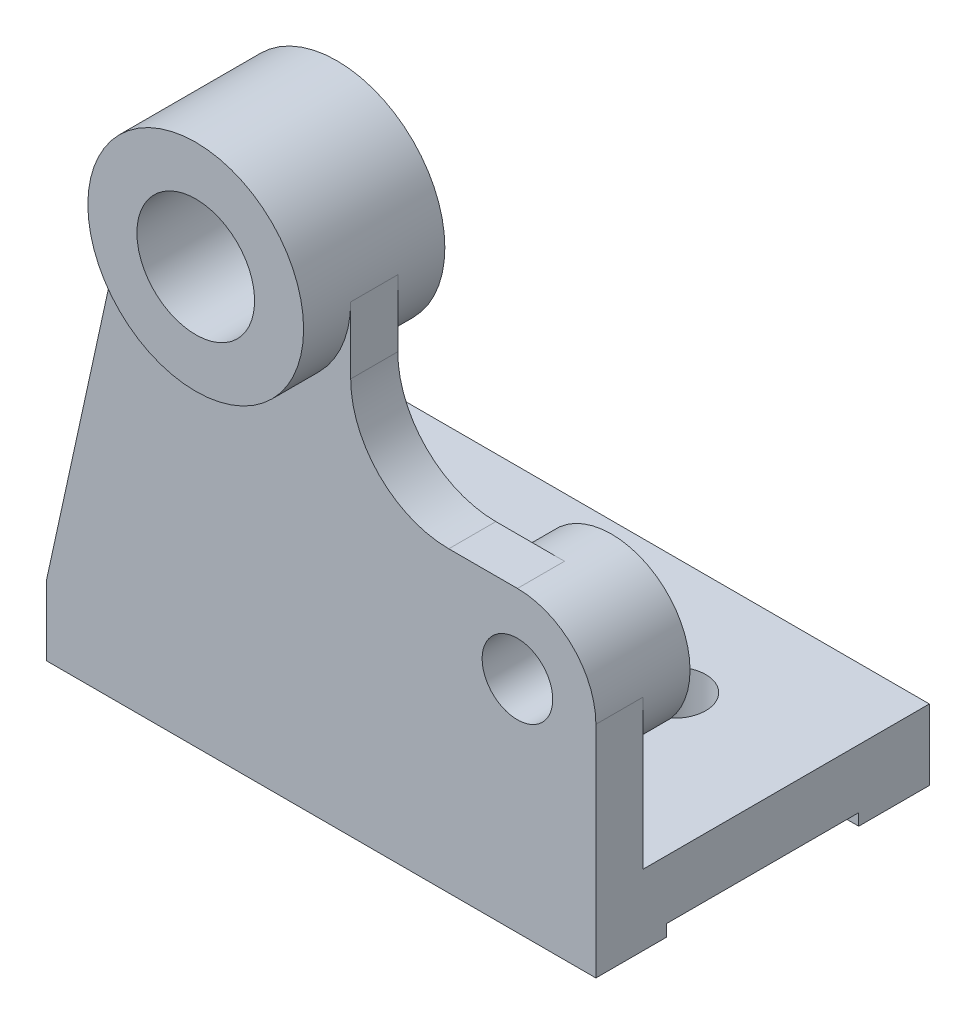
ISO-10303-21;
HEADER;
FILE_DESCRIPTION(('STEP AP214'),'2;1');
FILE_NAME('part.step','',(''),(''),'','','');
FILE_SCHEMA(('AUTOMOTIVE_DESIGN { 1 0 10303 214 1 1 1 1 }'));
ENDSEC;
DATA;
#1=APPLICATION_CONTEXT('core data for automotive mechanical design processes');
#2=APPLICATION_PROTOCOL_DEFINITION('international standard','automotive_design',2000,#1);
#3=PRODUCT_CONTEXT('',#1,'mechanical');
#4=PRODUCT('Part','Part','',(#3));
#5=PRODUCT_RELATED_PRODUCT_CATEGORY('part','',(#4));
#6=PRODUCT_DEFINITION_FORMATION('','',#4);
#7=PRODUCT_DEFINITION_CONTEXT('part definition',#1,'design');
#8=PRODUCT_DEFINITION('design','',#6,#7);
#9=PRODUCT_DEFINITION_SHAPE('','',#8);
#10=(LENGTH_UNIT() NAMED_UNIT(*) SI_UNIT(.MILLI.,.METRE.));
#11=(NAMED_UNIT(*) PLANE_ANGLE_UNIT() SI_UNIT($,.RADIAN.));
#12=(NAMED_UNIT(*) SI_UNIT($,.STERADIAN.) SOLID_ANGLE_UNIT());
#13=UNCERTAINTY_MEASURE_WITH_UNIT(LENGTH_MEASURE(1.E-05),#10,'distance_accuracy_value','');
#14=(GEOMETRIC_REPRESENTATION_CONTEXT(3) GLOBAL_UNCERTAINTY_ASSIGNED_CONTEXT((#13)) GLOBAL_UNIT_ASSIGNED_CONTEXT((#10,
#11,#12)) REPRESENTATION_CONTEXT('',''));
#15=CARTESIAN_POINT('',(0.,0.,0.));
#16=DIRECTION('',(0.,0.,1.));
#17=DIRECTION('',(1.,0.,0.));
#18=AXIS2_PLACEMENT_3D('',#15,#16,#17);
#19=CARTESIAN_POINT('',(70.,9.,42.5));
#20=DIRECTION('',(0.,-1.,0.));
#21=DIRECTION('',(0.,0.,-1.));
#22=AXIS2_PLACEMENT_3D('',#19,#20,#21);
#23=PLANE('',#22);
#24=CARTESIAN_POINT('',(-35.,9.00000000000001,-12.5));
#25=DIRECTION('',(0.,-1.,0.));
#26=DIRECTION('',(0.,0.,-1.));
#27=AXIS2_PLACEMENT_3D('',#24,#25,#26);
#28=CIRCLE('',#27,8.);
#29=CARTESIAN_POINT('',(-35.,9.00000000000001,-20.5));
#30=VERTEX_POINT('',#29);
#31=EDGE_CURVE('E269',#30,#30,#28,.F.);
#32=ORIENTED_EDGE('',*,*,#31,.F.);
#33=EDGE_LOOP('',(#32));
#34=FACE_BOUND('',#33,.T.);
#35=CARTESIAN_POINT('',(35.,9.00000000000001,-12.5));
#36=DIRECTION('',(0.,-1.,0.));
#37=DIRECTION('',(0.,0.,-1.));
#38=AXIS2_PLACEMENT_3D('',#35,#36,#37);
#39=CIRCLE('',#38,8.);
#40=CARTESIAN_POINT('',(35.,9.00000000000001,-20.5));
#41=VERTEX_POINT('',#40);
#42=EDGE_CURVE('E272',#41,#41,#39,.F.);
#43=ORIENTED_EDGE('',*,*,#42,.F.);
#44=EDGE_LOOP('',(#43));
#45=FACE_BOUND('',#44,.T.);
#46=DIRECTION('',(-1.,0.,0.));
#47=VECTOR('',#46,1.);
#48=CARTESIAN_POINT('',(70.,9.,30.5));
#49=LINE('',#48,#47);
#50=CARTESIAN_POINT('',(70.,9.,30.5));
#51=VERTEX_POINT('',#50);
#52=CARTESIAN_POINT('',(-70.,9.,30.5));
#53=VERTEX_POINT('',#52);
#54=EDGE_CURVE('E57',#51,#53,#49,.T.);
#55=ORIENTED_EDGE('',*,*,#54,.F.);
#56=DIRECTION('',(0.,0.,1.));
#57=VECTOR('',#56,1.);
#58=CARTESIAN_POINT('',(70.,9.,42.5));
#59=LINE('',#58,#57);
#60=CARTESIAN_POINT('',(70.,9.,-42.5));
#61=VERTEX_POINT('',#60);
#62=EDGE_CURVE('E105',#61,#51,#59,.T.);
#63=ORIENTED_EDGE('',*,*,#62,.F.);
#64=DIRECTION('',(-1.,0.,0.));
#65=VECTOR('',#64,1.);
#66=CARTESIAN_POINT('',(70.,9.,-42.5));
#67=LINE('',#66,#65);
#68=CARTESIAN_POINT('',(-70.,9.,-42.5));
#69=VERTEX_POINT('',#68);
#70=EDGE_CURVE('E11',#61,#69,#67,.T.);
#71=ORIENTED_EDGE('',*,*,#70,.T.);
#72=DIRECTION('',(0.,0.,1.));
#73=VECTOR('',#72,1.);
#74=CARTESIAN_POINT('',(-70.,9.,42.5));
#75=LINE('',#74,#73);
#76=EDGE_CURVE('E150',#69,#53,#75,.T.);
#77=ORIENTED_EDGE('',*,*,#76,.T.);
#78=EDGE_LOOP('',(#55,#63,#71,#77));
#79=FACE_BOUND('',#78,.T.);
#80=ADVANCED_FACE('F41',(#34,#45,#79),#23,.F.);
#81=CARTESIAN_POINT('',(70.,-9.,-42.5));
#82=DIRECTION('',(0.,0.,1.));
#83=DIRECTION('',(1.,0.,0.));
#84=AXIS2_PLACEMENT_3D('',#81,#82,#83);
#85=PLANE('',#84);
#86=DIRECTION('',(0.,1.,0.));
#87=VECTOR('',#86,1.);
#88=CARTESIAN_POINT('',(-70.,-9.,-42.5));
#89=LINE('',#88,#87);
#90=CARTESIAN_POINT('',(-70.,-9.,-42.5));
#91=VERTEX_POINT('',#90);
#92=EDGE_CURVE('E145',#91,#69,#89,.T.);
#93=ORIENTED_EDGE('',*,*,#92,.T.);
#94=ORIENTED_EDGE('',*,*,#70,.F.);
#95=DIRECTION('',(0.,1.,0.));
#96=VECTOR('',#95,1.);
#97=CARTESIAN_POINT('',(70.,-9.,-42.5));
#98=LINE('',#97,#96);
#99=CARTESIAN_POINT('',(70.,-9.,-42.5));
#100=VERTEX_POINT('',#99);
#101=EDGE_CURVE('E159',#100,#61,#98,.T.);
#102=ORIENTED_EDGE('',*,*,#101,.F.);
#103=DIRECTION('',(-1.,0.,0.));
#104=VECTOR('',#103,1.);
#105=CARTESIAN_POINT('',(70.,-9.,-42.5));
#106=LINE('',#105,#104);
#107=EDGE_CURVE('E139',#100,#91,#106,.T.);
#108=ORIENTED_EDGE('',*,*,#107,.T.);
#109=EDGE_LOOP('',(#93,#94,#102,#108));
#110=FACE_BOUND('',#109,.T.);
#111=ADVANCED_FACE('F43',(#110),#85,.F.);
#112=CARTESIAN_POINT('',(70.,-9.,42.5));
#113=DIRECTION('',(0.,0.,-1.));
#114=DIRECTION('',(-1.,0.,0.));
#115=AXIS2_PLACEMENT_3D('',#112,#113,#114);
#116=PLANE('',#115);
#117=DIRECTION('',(0.,-1.,0.));
#118=VECTOR('',#117,1.);
#119=CARTESIAN_POINT('',(7.5,109.,42.5));
#120=LINE('',#119,#118);
#121=CARTESIAN_POINT('',(7.49999999999999,109.,42.5));
#122=VERTEX_POINT('',#121);
#123=CARTESIAN_POINT('',(7.49999999999999,92.,42.5));
#124=VERTEX_POINT('',#123);
#125=EDGE_CURVE('E220',#122,#124,#120,.T.);
#126=ORIENTED_EDGE('',*,*,#125,.F.);
#127=CARTESIAN_POINT('',(-20.,109.,42.5));
#128=DIRECTION('',(0.,0.,-1.));
#129=DIRECTION('',(-1.,0.,0.));
#130=AXIS2_PLACEMENT_3D('',#127,#128,#129);
#131=CIRCLE('',#130,27.5);
#132=CARTESIAN_POINT('',(-46.8660884818626,114.870544240931,42.5));
#133=VERTEX_POINT('',#132);
#134=EDGE_CURVE('E248',#122,#133,#131,.T.);
#135=ORIENTED_EDGE('',*,*,#134,.T.);
#136=DIRECTION('',(0.213474336033865,0.97694867206773,0.));
#137=VECTOR('',#136,1.);
#138=CARTESIAN_POINT('',(-70.,9.,42.5));
#139=LINE('',#138,#137);
#140=CARTESIAN_POINT('',(-70.,9.,42.5));
#141=VERTEX_POINT('',#140);
#142=EDGE_CURVE('E219',#141,#133,#139,.T.);
#143=ORIENTED_EDGE('',*,*,#142,.F.);
#144=DIRECTION('',(0.,-1.,0.));
#145=VECTOR('',#144,1.);
#146=CARTESIAN_POINT('',(-70.,-9.,42.5));
#147=LINE('',#146,#145);
#148=CARTESIAN_POINT('',(-70.,-9.,42.5));
#149=VERTEX_POINT('',#148);
#150=EDGE_CURVE('E147',#141,#149,#147,.T.);
#151=ORIENTED_EDGE('',*,*,#150,.T.);
#152=DIRECTION('',(-1.,0.,0.));
#153=VECTOR('',#152,1.);
#154=CARTESIAN_POINT('',(70.,-9.,42.5));
#155=LINE('',#154,#153);
#156=CARTESIAN_POINT('',(70.,-9.,42.5));
#157=VERTEX_POINT('',#156);
#158=EDGE_CURVE('E47',#157,#149,#155,.T.);
#159=ORIENTED_EDGE('',*,*,#158,.F.);
#160=DIRECTION('',(0.,-1.,0.));
#161=VECTOR('',#160,1.);
#162=CARTESIAN_POINT('',(70.,-9.,42.5));
#163=LINE('',#162,#161);
#164=CARTESIAN_POINT('',(70.,47.,42.5));
#165=VERTEX_POINT('',#164);
#166=EDGE_CURVE('E184',#165,#157,#163,.T.);
#167=ORIENTED_EDGE('',*,*,#166,.F.);
#168=CARTESIAN_POINT('',(50.,47.,42.5));
#169=DIRECTION('',(0.,0.,-1.));
#170=DIRECTION('',(-1.,0.,0.));
#171=AXIS2_PLACEMENT_3D('',#168,#169,#170);
#172=CIRCLE('',#171,20.);
#173=CARTESIAN_POINT('',(50.,67.,42.5));
#174=VERTEX_POINT('',#173);
#175=EDGE_CURVE('E224',#174,#165,#172,.T.);
#176=ORIENTED_EDGE('',*,*,#175,.F.);
#177=DIRECTION('',(1.,0.,0.));
#178=VECTOR('',#177,1.);
#179=CARTESIAN_POINT('',(50.,67.,42.5));
#180=LINE('',#179,#178);
#181=CARTESIAN_POINT('',(32.5,67.,42.5));
#182=VERTEX_POINT('',#181);
#183=EDGE_CURVE('E209',#182,#174,#180,.T.);
#184=ORIENTED_EDGE('',*,*,#183,.F.);
#185=CARTESIAN_POINT('',(32.5,92.,42.5));
#186=DIRECTION('',(0.,0.,1.));
#187=DIRECTION('',(-1.,0.,0.));
#188=AXIS2_PLACEMENT_3D('',#185,#186,#187);
#189=CIRCLE('',#188,25.);
#190=EDGE_CURVE('E212',#124,#182,#189,.T.);
#191=ORIENTED_EDGE('',*,*,#190,.F.);
#192=EDGE_LOOP('',(#126,#135,#143,#151,#159,#167,#176,#184,#191));
#193=FACE_BOUND('',#192,.T.);
#194=CARTESIAN_POINT('',(50.,47.,42.5));
#195=DIRECTION('',(0.,0.,-1.));
#196=DIRECTION('',(-1.,0.,0.));
#197=AXIS2_PLACEMENT_3D('',#194,#195,#196);
#198=CIRCLE('',#197,9.);
#199=CARTESIAN_POINT('',(41.,47.,42.5));
#200=VERTEX_POINT('',#199);
#201=EDGE_CURVE('E227',#200,#200,#198,.T.);
#202=ORIENTED_EDGE('',*,*,#201,.T.);
#203=EDGE_LOOP('',(#202));
#204=FACE_BOUND('',#203,.T.);
#205=ADVANCED_FACE('F302',(#193,#204),#116,.F.);
#206=CARTESIAN_POINT('',(70.,-9.,42.5));
#207=DIRECTION('',(0.,1.,0.));
#208=DIRECTION('',(0.,0.,1.));
#209=AXIS2_PLACEMENT_3D('',#206,#207,#208);
#210=PLANE('',#209);
#211=DIRECTION('',(0.,0.,-1.));
#212=VECTOR('',#211,1.);
#213=CARTESIAN_POINT('',(-70.,-9.,42.5));
#214=LINE('',#213,#212);
#215=CARTESIAN_POINT('',(-70.,-9.,24.5));
#216=VERTEX_POINT('',#215);
#217=EDGE_CURVE('E155',#149,#216,#214,.T.);
#218=ORIENTED_EDGE('',*,*,#217,.T.);
#219=DIRECTION('',(-1.,0.,0.));
#220=VECTOR('',#219,1.);
#221=CARTESIAN_POINT('',(70.,-9.,24.5));
#222=LINE('',#221,#220);
#223=CARTESIAN_POINT('',(70.,-9.,24.5));
#224=VERTEX_POINT('',#223);
#225=EDGE_CURVE('E163',#224,#216,#222,.T.);
#226=ORIENTED_EDGE('',*,*,#225,.F.);
#227=DIRECTION('',(0.,0.,-1.));
#228=VECTOR('',#227,1.);
#229=CARTESIAN_POINT('',(70.,-9.,42.5));
#230=LINE('',#229,#228);
#231=EDGE_CURVE('E175',#157,#224,#230,.T.);
#232=ORIENTED_EDGE('',*,*,#231,.F.);
#233=ORIENTED_EDGE('',*,*,#158,.T.);
#234=EDGE_LOOP('',(#218,#226,#232,#233));
#235=FACE_BOUND('',#234,.T.);
#236=ADVANCED_FACE('F172',(#235),#210,.F.);
#237=CARTESIAN_POINT('',(70.,-9.,24.5));
#238=DIRECTION('',(0.,0.,1.));
#239=DIRECTION('',(1.,0.,0.));
#240=AXIS2_PLACEMENT_3D('',#237,#238,#239);
#241=PLANE('',#240);
#242=DIRECTION('',(0.,1.,0.));
#243=VECTOR('',#242,1.);
#244=CARTESIAN_POINT('',(-70.,-9.,24.5));
#245=LINE('',#244,#243);
#246=CARTESIAN_POINT('',(-70.,-6.,24.5));
#247=VERTEX_POINT('',#246);
#248=EDGE_CURVE('E152',#216,#247,#245,.T.);
#249=ORIENTED_EDGE('',*,*,#248,.T.);
#250=DIRECTION('',(-1.,0.,0.));
#251=VECTOR('',#250,1.);
#252=CARTESIAN_POINT('',(70.,-6.,24.5));
#253=LINE('',#252,#251);
#254=CARTESIAN_POINT('',(70.,-6.,24.5));
#255=VERTEX_POINT('',#254);
#256=EDGE_CURVE('E133',#255,#247,#253,.T.);
#257=ORIENTED_EDGE('',*,*,#256,.F.);
#258=DIRECTION('',(0.,1.,0.));
#259=VECTOR('',#258,1.);
#260=CARTESIAN_POINT('',(70.,-9.,24.5));
#261=LINE('',#260,#259);
#262=EDGE_CURVE('E123',#224,#255,#261,.T.);
#263=ORIENTED_EDGE('',*,*,#262,.F.);
#264=ORIENTED_EDGE('',*,*,#225,.T.);
#265=EDGE_LOOP('',(#249,#257,#263,#264));
#266=FACE_BOUND('',#265,.T.);
#267=ADVANCED_FACE('F181',(#266),#241,.F.);
#268=CARTESIAN_POINT('',(70.,-6.,24.5));
#269=DIRECTION('',(0.,1.,0.));
#270=DIRECTION('',(0.,0.,1.));
#271=AXIS2_PLACEMENT_3D('',#268,#269,#270);
#272=PLANE('',#271);
#273=CARTESIAN_POINT('',(-35.,-6.,-12.5));
#274=DIRECTION('',(0.,1.,0.));
#275=DIRECTION('',(0.,0.,1.));
#276=AXIS2_PLACEMENT_3D('',#273,#274,#275);
#277=CIRCLE('',#276,8.);
#278=CARTESIAN_POINT('',(-35.,-6.,-4.49999999999998));
#279=VERTEX_POINT('',#278);
#280=EDGE_CURVE('E277',#279,#279,#277,.F.);
#281=ORIENTED_EDGE('',*,*,#280,.F.);
#282=EDGE_LOOP('',(#281));
#283=FACE_BOUND('',#282,.T.);
#284=CARTESIAN_POINT('',(35.,-6.,-12.5));
#285=DIRECTION('',(0.,1.,0.));
#286=DIRECTION('',(0.,0.,1.));
#287=AXIS2_PLACEMENT_3D('',#284,#285,#286);
#288=CIRCLE('',#287,8.);
#289=CARTESIAN_POINT('',(35.,-6.,-4.49999999999998));
#290=VERTEX_POINT('',#289);
#291=EDGE_CURVE('E280',#290,#290,#288,.F.);
#292=ORIENTED_EDGE('',*,*,#291,.F.);
#293=EDGE_LOOP('',(#292));
#294=FACE_BOUND('',#293,.T.);
#295=DIRECTION('',(0.,0.,-1.));
#296=VECTOR('',#295,1.);
#297=CARTESIAN_POINT('',(-70.,-6.,24.5));
#298=LINE('',#297,#296);
#299=CARTESIAN_POINT('',(-70.,-6.,-24.5));
#300=VERTEX_POINT('',#299);
#301=EDGE_CURVE('E134',#247,#300,#298,.T.);
#302=ORIENTED_EDGE('',*,*,#301,.T.);
#303=DIRECTION('',(-1.,0.,0.));
#304=VECTOR('',#303,1.);
#305=CARTESIAN_POINT('',(70.,-6.,-24.5));
#306=LINE('',#305,#304);
#307=CARTESIAN_POINT('',(70.,-6.,-24.5));
#308=VERTEX_POINT('',#307);
#309=EDGE_CURVE('E129',#308,#300,#306,.T.);
#310=ORIENTED_EDGE('',*,*,#309,.F.);
#311=DIRECTION('',(0.,0.,-1.));
#312=VECTOR('',#311,1.);
#313=CARTESIAN_POINT('',(70.,-6.,24.5));
#314=LINE('',#313,#312);
#315=EDGE_CURVE('E117',#255,#308,#314,.T.);
#316=ORIENTED_EDGE('',*,*,#315,.F.);
#317=ORIENTED_EDGE('',*,*,#256,.T.);
#318=EDGE_LOOP('',(#302,#310,#316,#317));
#319=FACE_BOUND('',#318,.T.);
#320=ADVANCED_FACE('F128',(#283,#294,#319),#272,.F.);
#321=CARTESIAN_POINT('',(70.,-6.,-24.5));
#322=DIRECTION('',(0.,0.,-1.));
#323=DIRECTION('',(0.,1.,0.));
#324=AXIS2_PLACEMENT_3D('',#321,#322,#323);
#325=PLANE('',#324);
#326=DIRECTION('',(0.,-1.,0.));
#327=VECTOR('',#326,1.);
#328=CARTESIAN_POINT('',(-70.,-6.,-24.5));
#329=LINE('',#328,#327);
#330=CARTESIAN_POINT('',(-70.,-9.,-24.5));
#331=VERTEX_POINT('',#330);
#332=EDGE_CURVE('E160',#300,#331,#329,.T.);
#333=ORIENTED_EDGE('',*,*,#332,.T.);
#334=DIRECTION('',(-1.,0.,0.));
#335=VECTOR('',#334,1.);
#336=CARTESIAN_POINT('',(70.,-9.,-24.5));
#337=LINE('',#336,#335);
#338=CARTESIAN_POINT('',(70.,-9.,-24.5));
#339=VERTEX_POINT('',#338);
#340=EDGE_CURVE('E136',#339,#331,#337,.T.);
#341=ORIENTED_EDGE('',*,*,#340,.F.);
#342=DIRECTION('',(0.,-1.,0.));
#343=VECTOR('',#342,1.);
#344=CARTESIAN_POINT('',(70.,-6.,-24.5));
#345=LINE('',#344,#343);
#346=EDGE_CURVE('E118',#308,#339,#345,.T.);
#347=ORIENTED_EDGE('',*,*,#346,.F.);
#348=ORIENTED_EDGE('',*,*,#309,.T.);
#349=EDGE_LOOP('',(#333,#341,#347,#348));
#350=FACE_BOUND('',#349,.T.);
#351=ADVANCED_FACE('F138',(#350),#325,.F.);
#352=CARTESIAN_POINT('',(70.,-9.,-24.5));
#353=DIRECTION('',(0.,1.,0.));
#354=DIRECTION('',(0.,0.,1.));
#355=AXIS2_PLACEMENT_3D('',#352,#353,#354);
#356=PLANE('',#355);
#357=DIRECTION('',(0.,0.,-1.));
#358=VECTOR('',#357,1.);
#359=CARTESIAN_POINT('',(-70.,-9.,-24.5));
#360=LINE('',#359,#358);
#361=EDGE_CURVE('E98',#331,#91,#360,.T.);
#362=ORIENTED_EDGE('',*,*,#361,.T.);
#363=ORIENTED_EDGE('',*,*,#107,.F.);
#364=DIRECTION('',(0.,0.,-1.));
#365=VECTOR('',#364,1.);
#366=CARTESIAN_POINT('',(70.,-9.,-24.5));
#367=LINE('',#366,#365);
#368=EDGE_CURVE('E63',#339,#100,#367,.T.);
#369=ORIENTED_EDGE('',*,*,#368,.F.);
#370=ORIENTED_EDGE('',*,*,#340,.T.);
#371=EDGE_LOOP('',(#362,#363,#369,#370));
#372=FACE_BOUND('',#371,.T.);
#373=ADVANCED_FACE('F316',(#372),#356,.F.);
#374=CARTESIAN_POINT('',(70.,0.,0.));
#375=DIRECTION('',(-1.,0.,0.));
#376=DIRECTION('',(0.,0.,1.));
#377=AXIS2_PLACEMENT_3D('',#374,#375,#376);
#378=PLANE('',#377);
#379=ORIENTED_EDGE('',*,*,#101,.T.);
#380=ORIENTED_EDGE('',*,*,#62,.T.);
#381=DIRECTION('',(0.,-1.,0.));
#382=VECTOR('',#381,1.);
#383=CARTESIAN_POINT('',(70.,47.,30.5));
#384=LINE('',#383,#382);
#385=CARTESIAN_POINT('',(70.,47.,30.5));
#386=VERTEX_POINT('',#385);
#387=EDGE_CURVE('E213',#386,#51,#384,.T.);
#388=ORIENTED_EDGE('',*,*,#387,.F.);
#389=DIRECTION('',(0.,0.,1.));
#390=VECTOR('',#389,1.);
#391=CARTESIAN_POINT('',(70.,47.,30.5));
#392=LINE('',#391,#390);
#393=EDGE_CURVE('E146',#386,#165,#392,.T.);
#394=ORIENTED_EDGE('',*,*,#393,.T.);
#395=ORIENTED_EDGE('',*,*,#166,.T.);
#396=ORIENTED_EDGE('',*,*,#231,.T.);
#397=ORIENTED_EDGE('',*,*,#262,.T.);
#398=ORIENTED_EDGE('',*,*,#315,.T.);
#399=ORIENTED_EDGE('',*,*,#346,.T.);
#400=ORIENTED_EDGE('',*,*,#368,.T.);
#401=EDGE_LOOP('',(#379,#380,#388,#394,#395,#396,#397,#398,#399,#400));
#402=FACE_BOUND('',#401,.T.);
#403=ADVANCED_FACE('F120',(#402),#378,.F.);
#404=CARTESIAN_POINT('',(-70.,0.,0.));
#405=DIRECTION('',(-1.,0.,0.));
#406=DIRECTION('',(0.,0.,1.));
#407=AXIS2_PLACEMENT_3D('',#404,#405,#406);
#408=PLANE('',#407);
#409=ORIENTED_EDGE('',*,*,#92,.F.);
#410=ORIENTED_EDGE('',*,*,#361,.F.);
#411=ORIENTED_EDGE('',*,*,#332,.F.);
#412=ORIENTED_EDGE('',*,*,#301,.F.);
#413=ORIENTED_EDGE('',*,*,#248,.F.);
#414=ORIENTED_EDGE('',*,*,#217,.F.);
#415=ORIENTED_EDGE('',*,*,#150,.F.);
#416=DIRECTION('',(0.,0.,1.));
#417=VECTOR('',#416,1.);
#418=CARTESIAN_POINT('',(-70.,9.,30.5));
#419=LINE('',#418,#417);
#420=EDGE_CURVE('E195',#53,#141,#419,.T.);
#421=ORIENTED_EDGE('',*,*,#420,.F.);
#422=ORIENTED_EDGE('',*,*,#76,.F.);
#423=EDGE_LOOP('',(#409,#410,#411,#412,#413,#414,#415,#421,#422));
#424=FACE_BOUND('',#423,.T.);
#425=ADVANCED_FACE('F177',(#424),#408,.T.);
#426=CARTESIAN_POINT('',(50.,47.,30.5));
#427=DIRECTION('',(0.,0.,-1.));
#428=DIRECTION('',(-1.,0.,0.));
#429=AXIS2_PLACEMENT_3D('',#426,#427,#428);
#430=PLANE('',#429);
#431=CARTESIAN_POINT('',(-20.,109.,30.5));
#432=DIRECTION('',(0.,0.,-1.));
#433=DIRECTION('',(-1.,0.,0.));
#434=AXIS2_PLACEMENT_3D('',#431,#432,#433);
#435=CIRCLE('',#434,27.5);
#436=CARTESIAN_POINT('',(7.49999999999999,109.,30.5));
#437=VERTEX_POINT('',#436);
#438=CARTESIAN_POINT('',(-46.8660884818626,114.870544240931,30.5));
#439=VERTEX_POINT('',#438);
#440=EDGE_CURVE('E254',#437,#439,#435,.T.);
#441=ORIENTED_EDGE('',*,*,#440,.F.);
#442=DIRECTION('',(0.,-1.,0.));
#443=VECTOR('',#442,1.);
#444=CARTESIAN_POINT('',(7.5,109.,30.5));
#445=LINE('',#444,#443);
#446=CARTESIAN_POINT('',(7.49999999999999,92.,30.5));
#447=VERTEX_POINT('',#446);
#448=EDGE_CURVE('E235',#437,#447,#445,.T.);
#449=ORIENTED_EDGE('',*,*,#448,.T.);
#450=CARTESIAN_POINT('',(32.5,92.,30.5));
#451=DIRECTION('',(0.,0.,1.));
#452=DIRECTION('',(-1.,0.,0.));
#453=AXIS2_PLACEMENT_3D('',#450,#451,#452);
#454=CIRCLE('',#453,25.);
#455=CARTESIAN_POINT('',(32.5,67.,30.5));
#456=VERTEX_POINT('',#455);
#457=EDGE_CURVE('E226',#447,#456,#454,.T.);
#458=ORIENTED_EDGE('',*,*,#457,.T.);
#459=DIRECTION('',(1.,0.,0.));
#460=VECTOR('',#459,1.);
#461=CARTESIAN_POINT('',(50.,67.,30.5));
#462=LINE('',#461,#460);
#463=CARTESIAN_POINT('',(50.,67.,30.5));
#464=VERTEX_POINT('',#463);
#465=EDGE_CURVE('E207',#456,#464,#462,.T.);
#466=ORIENTED_EDGE('',*,*,#465,.T.);
#467=CARTESIAN_POINT('',(50.,47.,30.5));
#468=DIRECTION('',(0.,0.,-1.));
#469=DIRECTION('',(-1.,0.,0.));
#470=AXIS2_PLACEMENT_3D('',#467,#468,#469);
#471=CIRCLE('',#470,20.);
#472=EDGE_CURVE('E241',#386,#464,#471,.T.);
#473=ORIENTED_EDGE('',*,*,#472,.F.);
#474=ORIENTED_EDGE('',*,*,#387,.T.);
#475=ORIENTED_EDGE('',*,*,#54,.T.);
#476=DIRECTION('',(0.213474336033865,0.97694867206773,0.));
#477=VECTOR('',#476,1.);
#478=CARTESIAN_POINT('',(-70.,9.,30.5));
#479=LINE('',#478,#477);
#480=EDGE_CURVE('E234',#53,#439,#479,.T.);
#481=ORIENTED_EDGE('',*,*,#480,.T.);
#482=EDGE_LOOP('',(#441,#449,#458,#466,#473,#474,#475,#481));
#483=FACE_BOUND('',#482,.T.);
#484=ADVANCED_FACE('F321',(#483),#430,.T.);
#485=CARTESIAN_POINT('',(50.,47.,30.5));
#486=DIRECTION('',(0.,0.,1.));
#487=DIRECTION('',(1.,0.,0.));
#488=AXIS2_PLACEMENT_3D('',#485,#486,#487);
#489=CYLINDRICAL_SURFACE('',#488,20.);
#490=ORIENTED_EDGE('',*,*,#175,.T.);
#491=ORIENTED_EDGE('',*,*,#393,.F.);
#492=ORIENTED_EDGE('',*,*,#472,.T.);
#493=DIRECTION('',(0.,0.,1.));
#494=VECTOR('',#493,1.);
#495=CARTESIAN_POINT('',(50.,67.,30.5));
#496=LINE('',#495,#494);
#497=EDGE_CURVE('E206',#464,#174,#496,.T.);
#498=ORIENTED_EDGE('',*,*,#497,.T.);
#499=EDGE_LOOP('',(#490,#491,#492,#498));
#500=FACE_BOUND('',#499,.T.);
#501=CARTESIAN_POINT('',(50.,47.,18.5));
#502=DIRECTION('',(0.,0.,-1.));
#503=DIRECTION('',(-1.,0.,0.));
#504=AXIS2_PLACEMENT_3D('',#501,#502,#503);
#505=CIRCLE('',#504,20.);
#506=CARTESIAN_POINT('',(30.,47.,18.5));
#507=VERTEX_POINT('',#506);
#508=EDGE_CURVE('E245',#507,#507,#505,.T.);
#509=ORIENTED_EDGE('',*,*,#508,.F.);
#510=EDGE_LOOP('',(#509));
#511=FACE_BOUND('',#510,.T.);
#512=ADVANCED_FACE('F322',(#500,#511),#489,.T.);
#513=CARTESIAN_POINT('',(-70.,9.,30.5));
#514=DIRECTION('',(0.97694867206773,-0.213474336033865,0.));
#515=DIRECTION('',(0.213474336033865,0.97694867206773,0.));
#516=AXIS2_PLACEMENT_3D('',#513,#514,#515);
#517=PLANE('',#516);
#518=ORIENTED_EDGE('',*,*,#142,.T.);
#519=DIRECTION('',(0.,0.,1.));
#520=VECTOR('',#519,1.);
#521=CARTESIAN_POINT('',(-46.8660884818626,114.870544240931,30.5));
#522=LINE('',#521,#520);
#523=EDGE_CURVE('E192',#439,#133,#522,.T.);
#524=ORIENTED_EDGE('',*,*,#523,.F.);
#525=ORIENTED_EDGE('',*,*,#480,.F.);
#526=ORIENTED_EDGE('',*,*,#420,.T.);
#527=EDGE_LOOP('',(#518,#524,#525,#526));
#528=FACE_BOUND('',#527,.T.);
#529=ADVANCED_FACE('F330',(#528),#517,.F.);
#530=CARTESIAN_POINT('',(-20.,109.,30.5));
#531=DIRECTION('',(0.,0.,1.));
#532=DIRECTION('',(1.,0.,0.));
#533=AXIS2_PLACEMENT_3D('',#530,#531,#532);
#534=CYLINDRICAL_SURFACE('',#533,27.5);
#535=ORIENTED_EDGE('',*,*,#523,.T.);
#536=ORIENTED_EDGE('',*,*,#134,.F.);
#537=DIRECTION('',(0.,0.,1.));
#538=VECTOR('',#537,1.);
#539=CARTESIAN_POINT('',(7.49999999999999,109.,30.5));
#540=LINE('',#539,#538);
#541=EDGE_CURVE('E197',#437,#122,#540,.T.);
#542=ORIENTED_EDGE('',*,*,#541,.F.);
#543=ORIENTED_EDGE('',*,*,#440,.T.);
#544=EDGE_LOOP('',(#535,#536,#542,#543));
#545=FACE_BOUND('',#544,.T.);
#546=CARTESIAN_POINT('',(-20.,109.,18.5));
#547=DIRECTION('',(0.,0.,-1.));
#548=DIRECTION('',(-1.,0.,0.));
#549=AXIS2_PLACEMENT_3D('',#546,#547,#548);
#550=CIRCLE('',#549,27.5);
#551=CARTESIAN_POINT('',(-47.5,109.,18.5));
#552=VERTEX_POINT('',#551);
#553=EDGE_CURVE('E262',#552,#552,#550,.T.);
#554=ORIENTED_EDGE('',*,*,#553,.F.);
#555=EDGE_LOOP('',(#554));
#556=FACE_BOUND('',#555,.T.);
#557=CARTESIAN_POINT('',(-20.,109.,54.5));
#558=DIRECTION('',(0.,0.,-1.));
#559=DIRECTION('',(-1.,0.,0.));
#560=AXIS2_PLACEMENT_3D('',#557,#558,#559);
#561=CIRCLE('',#560,27.5);
#562=CARTESIAN_POINT('',(-47.5,109.,54.5));
#563=VERTEX_POINT('',#562);
#564=EDGE_CURVE('E256',#563,#563,#561,.T.);
#565=ORIENTED_EDGE('',*,*,#564,.T.);
#566=EDGE_LOOP('',(#565));
#567=FACE_BOUND('',#566,.T.);
#568=ADVANCED_FACE('F332',(#545,#556,#567),#534,.T.);
#569=CARTESIAN_POINT('',(7.5,109.,30.5));
#570=DIRECTION('',(-1.,0.,0.));
#571=DIRECTION('',(0.,-1.,0.));
#572=AXIS2_PLACEMENT_3D('',#569,#570,#571);
#573=PLANE('',#572);
#574=ORIENTED_EDGE('',*,*,#125,.T.);
#575=DIRECTION('',(0.,0.,1.));
#576=VECTOR('',#575,1.);
#577=CARTESIAN_POINT('',(7.49999999999999,92.,30.5));
#578=LINE('',#577,#576);
#579=EDGE_CURVE('E199',#447,#124,#578,.T.);
#580=ORIENTED_EDGE('',*,*,#579,.F.);
#581=ORIENTED_EDGE('',*,*,#448,.F.);
#582=ORIENTED_EDGE('',*,*,#541,.T.);
#583=EDGE_LOOP('',(#574,#580,#581,#582));
#584=FACE_BOUND('',#583,.T.);
#585=ADVANCED_FACE('F333',(#584),#573,.F.);
#586=CARTESIAN_POINT('',(32.5,92.,30.5));
#587=DIRECTION('',(0.,0.,1.));
#588=DIRECTION('',(1.,0.,0.));
#589=AXIS2_PLACEMENT_3D('',#586,#587,#588);
#590=CYLINDRICAL_SURFACE('',#589,25.);
#591=ORIENTED_EDGE('',*,*,#190,.T.);
#592=DIRECTION('',(0.,0.,1.));
#593=VECTOR('',#592,1.);
#594=CARTESIAN_POINT('',(32.5,67.,30.5));
#595=LINE('',#594,#593);
#596=EDGE_CURVE('E201',#456,#182,#595,.T.);
#597=ORIENTED_EDGE('',*,*,#596,.F.);
#598=ORIENTED_EDGE('',*,*,#457,.F.);
#599=ORIENTED_EDGE('',*,*,#579,.T.);
#600=EDGE_LOOP('',(#591,#597,#598,#599));
#601=FACE_BOUND('',#600,.T.);
#602=ADVANCED_FACE('F336',(#601),#590,.F.);
#603=CARTESIAN_POINT('',(50.,67.,30.5));
#604=DIRECTION('',(0.,-1.,0.));
#605=DIRECTION('',(0.,0.,-1.));
#606=AXIS2_PLACEMENT_3D('',#603,#604,#605);
#607=PLANE('',#606);
#608=ORIENTED_EDGE('',*,*,#183,.T.);
#609=ORIENTED_EDGE('',*,*,#497,.F.);
#610=ORIENTED_EDGE('',*,*,#465,.F.);
#611=ORIENTED_EDGE('',*,*,#596,.T.);
#612=EDGE_LOOP('',(#608,#609,#610,#611));
#613=FACE_BOUND('',#612,.T.);
#614=ADVANCED_FACE('F343',(#613),#607,.F.);
#615=CARTESIAN_POINT('',(50.,47.,30.5));
#616=DIRECTION('',(0.,0.,1.));
#617=DIRECTION('',(1.,0.,0.));
#618=AXIS2_PLACEMENT_3D('',#615,#616,#617);
#619=CYLINDRICAL_SURFACE('',#618,9.);
#620=ORIENTED_EDGE('',*,*,#201,.F.);
#621=EDGE_LOOP('',(#620));
#622=FACE_BOUND('',#621,.T.);
#623=CARTESIAN_POINT('',(50.,47.,18.5));
#624=DIRECTION('',(0.,0.,-1.));
#625=DIRECTION('',(-1.,0.,0.));
#626=AXIS2_PLACEMENT_3D('',#623,#624,#625);
#627=CIRCLE('',#626,9.);
#628=CARTESIAN_POINT('',(41.,47.,18.5));
#629=VERTEX_POINT('',#628);
#630=EDGE_CURVE('E250',#629,#629,#627,.F.);
#631=ORIENTED_EDGE('',*,*,#630,.F.);
#632=EDGE_LOOP('',(#631));
#633=FACE_BOUND('',#632,.T.);
#634=ADVANCED_FACE('F350',(#622,#633),#619,.F.);
#635=CARTESIAN_POINT('',(0.,0.,18.5));
#636=DIRECTION('',(0.,0.,-1.));
#637=DIRECTION('',(-1.,0.,0.));
#638=AXIS2_PLACEMENT_3D('',#635,#636,#637);
#639=PLANE('',#638);
#640=ORIENTED_EDGE('',*,*,#630,.T.);
#641=EDGE_LOOP('',(#640));
#642=FACE_BOUND('',#641,.T.);
#643=ORIENTED_EDGE('',*,*,#508,.T.);
#644=EDGE_LOOP('',(#643));
#645=FACE_BOUND('',#644,.T.);
#646=ADVANCED_FACE('F351',(#642,#645),#639,.T.);
#647=CARTESIAN_POINT('',(0.,0.,18.5));
#648=DIRECTION('',(0.,0.,-1.));
#649=DIRECTION('',(-1.,0.,0.));
#650=AXIS2_PLACEMENT_3D('',#647,#648,#649);
#651=PLANE('',#650);
#652=CARTESIAN_POINT('',(-20.,109.,18.5));
#653=DIRECTION('',(0.,0.,-1.));
#654=DIRECTION('',(-1.,0.,0.));
#655=AXIS2_PLACEMENT_3D('',#652,#653,#654);
#656=CIRCLE('',#655,15.);
#657=CARTESIAN_POINT('',(-35.,109.,18.5));
#658=VERTEX_POINT('',#657);
#659=EDGE_CURVE('E270',#658,#658,#656,.F.);
#660=ORIENTED_EDGE('',*,*,#659,.T.);
#661=EDGE_LOOP('',(#660));
#662=FACE_BOUND('',#661,.T.);
#663=ORIENTED_EDGE('',*,*,#553,.T.);
#664=EDGE_LOOP('',(#663));
#665=FACE_BOUND('',#664,.T.);
#666=ADVANCED_FACE('F357',(#662,#665),#651,.T.);
#667=CARTESIAN_POINT('',(-20.,109.,30.5));
#668=DIRECTION('',(0.,0.,1.));
#669=DIRECTION('',(1.,0.,0.));
#670=AXIS2_PLACEMENT_3D('',#667,#668,#669);
#671=CYLINDRICAL_SURFACE('',#670,15.);
#672=ORIENTED_EDGE('',*,*,#659,.F.);
#673=EDGE_LOOP('',(#672));
#674=FACE_BOUND('',#673,.T.);
#675=CARTESIAN_POINT('',(-20.,109.,54.5));
#676=DIRECTION('',(0.,0.,-1.));
#677=DIRECTION('',(-1.,0.,0.));
#678=AXIS2_PLACEMENT_3D('',#675,#676,#677);
#679=CIRCLE('',#678,15.);
#680=CARTESIAN_POINT('',(-35.,109.,54.5));
#681=VERTEX_POINT('',#680);
#682=EDGE_CURVE('E261',#681,#681,#679,.F.);
#683=ORIENTED_EDGE('',*,*,#682,.T.);
#684=EDGE_LOOP('',(#683));
#685=FACE_BOUND('',#684,.T.);
#686=ADVANCED_FACE('F356',(#674,#685),#671,.F.);
#687=CARTESIAN_POINT('',(0.,0.,54.5));
#688=DIRECTION('',(0.,0.,-1.));
#689=DIRECTION('',(-1.,0.,0.));
#690=AXIS2_PLACEMENT_3D('',#687,#688,#689);
#691=PLANE('',#690);
#692=ORIENTED_EDGE('',*,*,#682,.F.);
#693=EDGE_LOOP('',(#692));
#694=FACE_BOUND('',#693,.T.);
#695=ORIENTED_EDGE('',*,*,#564,.F.);
#696=EDGE_LOOP('',(#695));
#697=FACE_BOUND('',#696,.T.);
#698=ADVANCED_FACE('F294',(#694,#697),#691,.F.);
#699=CARTESIAN_POINT('',(35.,136.5,-12.5));
#700=DIRECTION('',(0.,-1.,0.));
#701=DIRECTION('',(0.,0.,-1.));
#702=AXIS2_PLACEMENT_3D('',#699,#700,#701);
#703=CYLINDRICAL_SURFACE('',#702,8.);
#704=ORIENTED_EDGE('',*,*,#291,.T.);
#705=EDGE_LOOP('',(#704));
#706=FACE_BOUND('',#705,.T.);
#707=ORIENTED_EDGE('',*,*,#42,.T.);
#708=EDGE_LOOP('',(#707));
#709=FACE_BOUND('',#708,.T.);
#710=ADVANCED_FACE('F292',(#706,#709),#703,.F.);
#711=CARTESIAN_POINT('',(-35.,136.5,-12.5));
#712=DIRECTION('',(0.,-1.,0.));
#713=DIRECTION('',(0.,0.,-1.));
#714=AXIS2_PLACEMENT_3D('',#711,#712,#713);
#715=CYLINDRICAL_SURFACE('',#714,8.);
#716=ORIENTED_EDGE('',*,*,#280,.T.);
#717=EDGE_LOOP('',(#716));
#718=FACE_BOUND('',#717,.T.);
#719=ORIENTED_EDGE('',*,*,#31,.T.);
#720=EDGE_LOOP('',(#719));
#721=FACE_BOUND('',#720,.T.);
#722=ADVANCED_FACE('F285',(#718,#721),#715,.F.);
#723=CLOSED_SHELL('',(#80,#111,#205,#236,#267,#320,#351,#373,#403,#425,#484,#512,#529,#568,#585,
#602,#614,#634,#646,#666,#686,#698,#710,#722));
#724=MANIFOLD_SOLID_BREP('B2',#723);
#725=ADVANCED_BREP_SHAPE_REPRESENTATION('',(#18,#724),#14);
#726=SHAPE_DEFINITION_REPRESENTATION(#9,#725);
ENDSEC;
END-ISO-10303-21;
